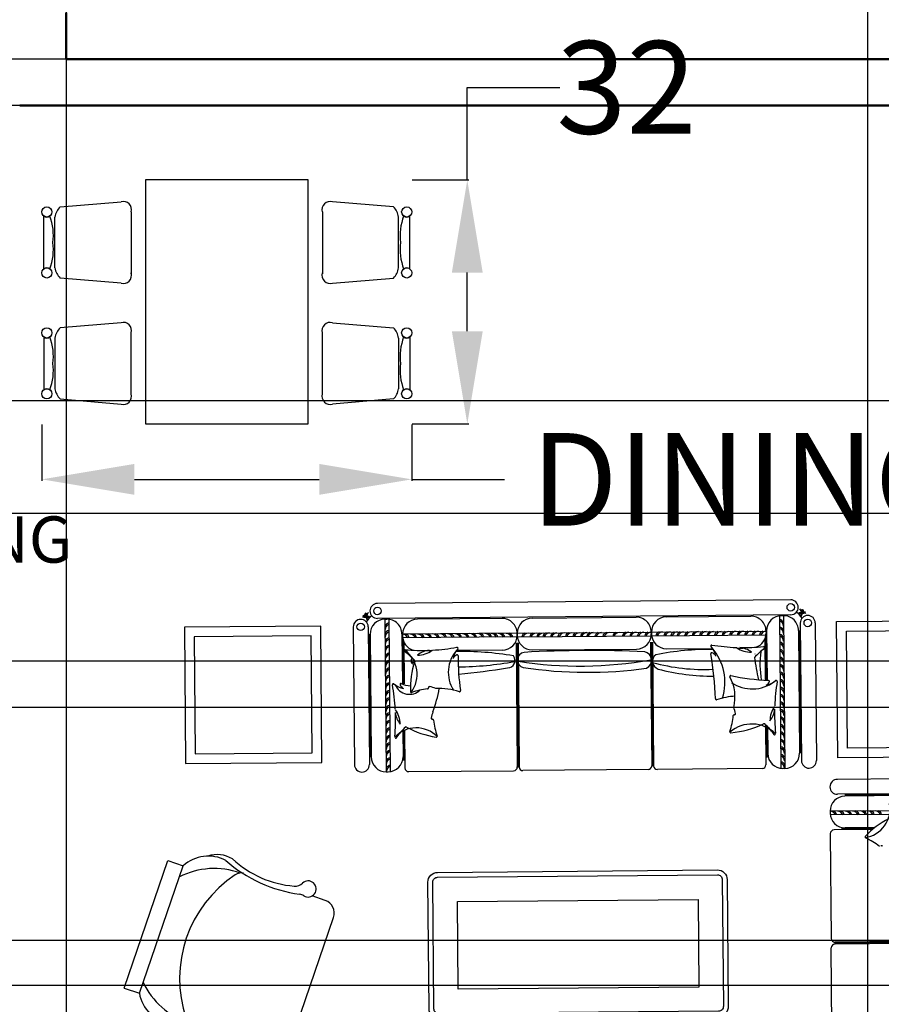
# Model space of a CAD drawing. Units: inches. Extents: x -77 to 516, y -119 to 536.
# Tile 8 of 11: x 224 to 335, y 159 to 287. Entities that reach past the tile are written whole.
import ezdxf

# ---------------------------------------------------------------- set-up
doc = ezdxf.new("R2010")
doc.units = ezdxf.units.IN
doc.header["$MEASUREMENT"] = 0
for name, color, linetype, lineweight in [('A-ANNO-DIMS', 2, 'Continuous', 18), ('A-AREA-IDEN', 170, 'Continuous', 25), ('furniture', 119, 'Continuous', 18), ('walls', 40, 'Continuous', 50)]:
    doc.layers.add(name, color=color, linetype=linetype, lineweight=lineweight)
doc.layers.add('FUR', color=42, linetype='Continuous')
doc.layers.add('ISLAK', color=6, linetype='Continuous')
doc.styles.get("Standard").update_dxf_attribs({"font": 'arial.ttf'})
doc.dimstyles.get("Standard").update_dxf_attribs({"dimtxt": 12, "dimasz": 12, "dimexe": 0.18, "dimexo": 0.0625, "dimgap": 0.09, "dimtad": 0, "dimtih": 1, "dimtoh": 1, "dimdec": 1, "dimzin": 0, "dimdsep": 46, "dimlunit": 4, "dimtxsty": 'Standard', "dimcen": 0.09, "dimadec": 0, "dimazin": 0, "dimtfac": 1, "dimtdec": 1, "dimtofl": 0, "dimtmove": 0, "dimatfit": 3, "dimfxl": 1, "dimtolj": 1, "dimtzin": 0, "dimarcsym": 0})

# ---------------------------------------------------------------- blocks, each defined once
blk = doc.blocks.new('A$C44A37715')
at = {"layer": 'FUR'}
for p, q in [((0.8644, 2.3252), (0.8644, 1.7873)), ((3.6462, 2.2614), (3.4159, 1.6094)), ((4.4156, 1.9896), (4.1853, 1.3376)), ((4.4938, 1.962), (4.4156, 1.9896)), ((4.4938, 1.962), (4.2635, 1.31)), ((0.2091, 1.7681), (0.8452, 1.7681)), ((0.2091, 1.7681), (0.8452, 1.7681)), ((0.2091, 1.7633), (0.8487, 1.7633)), ((0.2091, 1.7585), (0.8452, 1.7585)), ((0.2103, 1.7681), (0.8452, 1.7681)), ((0.8644, 1.2015), (0.8644, 1.7393)), ((3.4581, 1.5211), (3.5245, 1.4977)), ((4.2635, 1.31), (4.1853, 1.3376)), ((0.6364, 1.1727), (0.7875, 1.1727)), ((0.6445, 1.1775), (0.807, 1.1775)), ((0.6483, 1.1823), (0.8452, 1.1823)), ((0.5573, 1.0862), (0.8644, 1.0862)), ((0.56, 1.1054), (0.8638, 1.1054)), ((0.8644, 1.0862), (0.8644, 1.0958)), ((0.1193, 0.9998), (0.8259, 0.9998)), ((0.1577, 1.0094), (0.7875, 1.0094)), ((0.1577, 1.0046), (0.7875, 1.0046)), ((0.8644, 0.9614), (0.8644, 0.9614)), ((0.1193, 0.923), (0.8259, 0.923)), ((0.1193, 0.923), (0.8259, 0.923)), ((0.9706, 0.8644), (0.9706, 0.8644)), ((1.0954, 0.8644), (1.105, 0.8644)), ((1.0954, 0.0809), (1.0954, 0.8644)), ((1.1146, 0.0815), (1.1146, 0.8638)), ((1.2107, 0.8644), (1.7485, 0.8644)), ((1.7965, 0.8644), (2.438, 0.8644)), ((3.0239, 0.8644), (2.486, 0.8644)), ((3.1199, 0.0815), (3.1199, 0.8638)), ((3.1391, 0.8644), (3.1295, 0.8644)), ((3.1391, 0.0809), (3.1391, 0.8644)), ((3.264, 0.8644), (3.264, 0.8644)), ((0.9322, 0.1193), (0.9322, 0.8259)), ((1.009, 0.1193), (1.009, 0.8259)), ((1.1915, 0.6395), (1.1915, 0.8452)), ((1.7677, 0.2103), (1.7677, 0.8452)), ((1.7725, 0.2103), (1.7725, 0.8485)), ((1.7773, 0.2103), (1.7773, 0.8452)), ((2.4572, 0.2091), (2.4572, 0.8452)), ((2.4572, 0.2091), (2.4572, 0.8452)), ((2.462, 0.2091), (2.462, 0.8487)), ((2.4668, 0.2091), (2.4668, 0.8452)), ((3.0431, 0.652), (3.0431, 0.8452)), ((3.2255, 0.1193), (3.2255, 0.8259)), ((3.3024, 0.1193), (3.3024, 0.8259)), ((3.3024, 0.1193), (3.3024, 0.8259)), ((1.0138, 0.1577), (1.0138, 0.7875)), ((1.0186, 0.1577), (1.0186, 0.7875)), ((1.1819, 0.6496), (1.1819, 0.7875)), ((1.1867, 0.6445), (1.1867, 0.807)), ((3.0479, 0.6542), (3.0479, 0.807)), ((3.0527, 0.6565), (3.0527, 0.7875)), ((3.2159, 0.1577), (3.2159, 0.7875)), ((3.2207, 0.1577), (3.2207, 0.7875)), ((1.1819, 0.1577), (1.1819, 0.413)), ((1.1867, 0.1845), (1.1867, 0.4135)), ((1.1915, 0.1995), (1.1915, 0.4138)), ((3.0431, 0.1995), (3.0431, 0.4138)), ((3.0479, 0.1845), (3.0479, 0.4135)), ((3.0527, 0.1577), (3.0527, 0.413)), ((1.3318, 0.2455), (1.3038, 0.2455)), ((1.696, 0.2455), (1.4606, 0.2455)), ((2.3845, 0.2455), (1.8504, 0.2455)), ((2.5386, 0.2455), (2.774, 0.2455)), ((2.9027, 0.2455), (2.9308, 0.2455)), ((1.185, 0.1591), (1.185, 0.1687)), ((1.7728, 0.1591), (1.185, 0.1591)), ((1.7722, 0.1783), (1.1856, 0.1783)), ((1.7728, 0.1591), (1.7728, 0.1687)), ((1.7735, 0.1591), (1.7735, 0.1687)), ((2.4613, 0.1591), (1.7735, 0.1591)), ((2.4607, 0.1783), (1.7741, 0.1783)), ((2.4613, 0.1591), (2.4613, 0.1687)), ((2.4613, 0.1591), (2.4613, 0.1687)), ((2.4617, 0.1591), (2.4617, 0.1687)), ((2.4617, 0.1591), (2.4617, 0.1687)), ((2.4617, 0.1591), (3.0495, 0.1591)), ((2.4623, 0.1783), (3.0489, 0.1783)), ((2.4631, 0.1591), (2.4631, 0.1687)), ((3.0495, 0.1591), (3.0495, 0.1687)), ((0.9706, 0.0809), (0.9706, 0.0809)), ((1.0572, 0.0768), (3.1773, 0.0768)), ((1.0954, 0.0809), (1.105, 0.0809)), ((1.696, 0.0822), (1.2619, 0.0822)), ((2.3845, 0.0822), (1.8504, 0.0822)), ((2.5386, 0.0822), (2.9727, 0.0822)), ((3.1391, 0.0809), (3.1295, 0.0809)), ((3.264, 0.0809), (3.264, 0.0809)), ((1.0188, 0.0384), (1.0188, 0.0384)), ((1.0572, 0), (3.1773, 0)), ((3.2157, 0.0384), (3.2157, 0.0384))]:
    blk.add_line(p, q, dxfattribs=at)
for points in [[(2.8805, 2.1325, -0.414214), (2.9305, 2.0825), (2.9305, 1.4325, -0.414214), (2.8805, 1.3825), (1.4454, 1.3825, -0.414214), (1.3954, 1.4325), (1.3954, 2.0825, -0.414214), (1.4454, 2.1325)], [(2.8805, 2.1075, -0.414214), (2.9055, 2.0825), (2.9055, 1.4325, -0.414214), (2.8805, 1.4075), (1.4454, 1.4075, -0.414214), (1.4204, 1.4325), (1.4204, 2.0825, -0.414214), (1.4454, 2.1075)]]:
    blk.add_lwpolyline(points, format="xyb", close=True, dxfattribs=at)
for points in [[(2.7805, 1.9825), (2.7805, 1.5325), (1.5454, 1.5325), (1.5454, 1.9825)], [(0.1226, 0.1134), (0.1226, 0.8134), (0.8226, 0.8134), (0.8226, 0.1134)], [(4.1685, 0.1134), (4.1685, 0.8134), (3.4685, 0.8134), (3.4685, 0.1134)], [(0.1726, 0.1634), (0.1726, 0.7634), (0.7726, 0.7634), (0.7726, 0.1634)], [(4.1185, 0.1634), (4.1185, 0.7634), (3.5185, 0.7634), (3.5185, 0.1634)]]:
    blk.add_lwpolyline(points, close=True, dxfattribs=at)
for centre in [(0.9706, 0.1193), (3.264, 0.1193), (1.0572, 0.0384), (3.1773, 0.0384)]:
    blk.add_circle(centre, 0.0192, dxfattribs=at)
for centre, radius, start, end in [((4.0372, 1.7694), 0.3939, 24.5429, 71.319), ((4.2282, 1.96), 0.1897, 8.9926, 80.0637), ((3.5673, 1.9225), 0.6416, 303.2315, 17.8639), ((0.8452, 1.7873), 0.0192, 270, 0), ((0.8452, 1.7393), 0.0192, 0, 90), ((3.4811, 1.5863), 0.0691, 160.5477, 250.5477), ((3.5455, 1.4619), 0.0415, 57.5813, 313.2014), ((3.5974, 1.5436), 0.0553, 237.5813, 261.4346), ((3.4801, 0.7648), 0.7323, 48.4002, 81.4346), ((3.6117, 1.3913), 0.0553, 85.1896, 133.2014), ((3.5729, 0.9298), 0.5185, 46.2014, 85.1896), ((3.8886, 1.4321), 0.0553, 256.3156, 303.2315), ((4.0292, 1.7466), 0.3939, 249.7764, 296.5525), ((4.0581, 1.4783), 0.1897, 241.0317, 312.1028), ((0.6012, 1.2702), 0.0048, 215.4865, 326.8671), ((0.8574, 1.5872), 0.4019, 232.3976, 244.3894), ((4.0123, 1.437), 0.1555, 238.7962, 287.4358), ((0.7061, 1.0752), 0.1492, 97.8738, 190.1124), ((0.3864, 1.4953), 0.4082, 295.8111, 316.9977), ((0.6816, 1.2205), 0.0048, 313.302, 64.3894), ((0.7875, 1.0958), 0.0768, 0, 90), ((0.8452, 1.2015), 0.0192, 270, 0), ((0.6245, 1.1094), 0.0245, 189.3902, 251.5618), ((0.6348, 1.1155), 0.0293, 200.1355, 268.1936), ((0.6629, 1.1094), 0.0245, 189.3902, 251.5618), ((0.6732, 1.1155), 0.0293, 200.1355, 268.1936), ((0.7013, 1.1094), 0.0245, 189.3902, 251.5618), ((0.7116, 1.1155), 0.0293, 200.1355, 268.1936), ((0.7397, 1.1094), 0.0245, 189.3902, 251.5618), ((0.75, 1.1155), 0.0293, 200.1355, 268.1936), ((0.7781, 1.1094), 0.0245, 189.3902, 251.5618), ((0.7885, 1.1155), 0.0293, 200.1355, 268.1936), ((0.7875, 1.0862), 0.0768, 270, 0), ((0.8165, 1.1094), 0.0245, 189.3902, 251.5618), ((0.8269, 1.1155), 0.0293, 200.1355, 268.1936), ((0.8549, 1.1094), 0.0245, 189.3902, 251.5618), ((0.8653, 1.1155), 0.0293, 200.1355, 268.1936), ((0.8259, 0.9614), 0.0384, 360, 90), ((0.8259, 0.9614), 0.0384, 270, 360), ((0.9706, 0.8259), 0.0384, 90, 180), ((0.9706, 0.8259), 0.0384, 0, 90), ((1.0954, 0.7875), 0.0768, 90, 180), ((1.1247, 0.8653), 0.0293, 181.8064, 249.8645), ((1.105, 0.7875), 0.0768, 0, 90), ((1.2107, 0.8452), 0.0192, 90, 180), ((1.7485, 0.8452), 0.0192, 360, 90), ((1.7965, 0.8452), 0.0192, 90, 180), ((2.438, 0.8452), 0.0192, 0, 90), ((2.486, 0.8452), 0.0192, 90, 180), ((3.0239, 0.8452), 0.0192, 360, 90), ((3.1295, 0.7875), 0.0768, 90, 180), ((3.1098, 0.8653), 0.0293, 290.1355, 358.1936), ((3.1391, 0.7875), 0.0768, 360, 90), ((3.264, 0.8259), 0.0384, 90, 180), ((3.264, 0.8259), 0.0384, 360, 90), ((1.1186, 0.8549), 0.0245, 198.4382, 260.6098), ((1.1247, 0.8269), 0.0293, 181.8064, 249.8645), ((1.1186, 0.8165), 0.0245, 198.4382, 260.6098), ((3.1159, 0.8549), 0.0245, 279.3902, 341.5618), ((3.1098, 0.8269), 0.0293, 290.1355, 358.1936), ((3.1159, 0.8165), 0.0245, 279.3902, 341.5618), ((1.1247, 0.7885), 0.0293, 181.8064, 249.8645), ((1.1186, 0.7781), 0.0245, 198.4382, 260.6098), ((3.1098, 0.7885), 0.0293, 290.1355, 358.1936), ((3.1159, 0.7781), 0.0245, 279.3902, 341.5618), ((1.1247, 0.75), 0.0293, 181.8064, 249.8645), ((1.1186, 0.7397), 0.0245, 198.4382, 260.6098), ((1.1247, 0.7116), 0.0293, 181.8064, 249.8645), ((3.1098, 0.75), 0.0293, 290.1355, 358.1936), ((3.1159, 0.7397), 0.0245, 279.3902, 341.5618), ((3.1098, 0.7116), 0.0293, 290.1355, 358.1936), ((1.1186, 0.7013), 0.0245, 198.4382, 260.6098), ((1.1247, 0.6732), 0.0293, 181.8064, 249.8645), ((0.1462, 0.589), 0.9988, 358.3824, 5.4148), ((1.1462, 0.6869), 0.0048, 335.526, 185.4148), ((1.2637, 0.8067), 0.1714, 224.534, 310.2675), ((1.8739, 1.2944), 0.9459, 220.1216, 224.1481), ((1.4224, 0.1376), 0.5445, 95.5708, 113.9077), ((1.7562, 0.5476), 0.4019, 161.7886, 173.7804), ((1.3698, 0.6747), 0.0048, 341.7886, 92.876), ((2.8815, 0.6843), 0.0048, 87.124, 198.2114), ((2.9845, 0.7907), 0.1505, 224.349, 316.1606), ((2.4952, 0.5572), 0.4019, 6.2196, 18.2114), ((2.8036, 0.2306), 0.4652, 60.481, 80.3238), ((2.3606, 1.2944), 0.9459, 315.8519, 319.8784), ((3.0883, 0.6869), 0.0048, 354.5852, 204.474), ((4.0883, 0.589), 0.9988, 174.5852, 181.6176), ((3.1159, 0.7013), 0.0245, 279.3902, 341.5618), ((3.1098, 0.6732), 0.0293, 290.1355, 358.1936), ((1.1186, 0.6629), 0.0245, 198.4382, 260.6098), ((1.1247, 0.6348), 0.0293, 181.8064, 249.8645), ((1.1186, 0.6245), 0.0245, 198.4382, 260.6098), ((1.2514, 0.5519), 0.1071, 140.4453, 175.2684), ((1.0442, 0.6194), 0.1246, 323.9244, 0.3374), ((1.1986, 0.639), 0.0048, 224.1481, 310.8342), ((3.0359, 0.639), 0.0048, 229.1658, 315.8519), ((2.9831, 0.5519), 0.1071, 4.7316, 39.5547), ((3.1903, 0.6194), 0.1246, 179.6626, 216.0756), ((3.1159, 0.6629), 0.0245, 279.3902, 341.5618), ((3.1098, 0.6348), 0.0293, 290.1355, 358.1936), ((3.1159, 0.6245), 0.0245, 279.3902, 341.5618), ((1.1247, 0.5964), 0.0293, 181.8064, 249.8645), ((1.1186, 0.586), 0.0245, 198.4382, 260.6098), ((1.1247, 0.558), 0.0293, 181.8064, 249.8645), ((1.3501, 0.5822), 0.0048, 79.311, 190.6915), ((1.5338, 0.6169), 0.1918, 190.6915, 200.5832), ((1.3518, 0.5916), 0.0048, 259.311, 353.7804), ((3.5654, 0.3102), 0.7132, 159.5737, 169.6301), ((2.8995, 0.6013), 0.0048, 186.2196, 280.689), ((2.7176, 0.6265), 0.1918, 339.4168, 349.3085), ((2.9013, 0.5918), 0.0048, 349.3085, 100.689), ((3.1098, 0.5964), 0.0293, 290.1355, 358.1936), ((3.1159, 0.586), 0.0245, 279.3902, 341.5618), ((3.1098, 0.558), 0.0293, 290.1355, 358.1936), ((1.1186, 0.5476), 0.0245, 198.4382, 260.6098), ((1.1247, 0.5195), 0.0293, 181.8064, 249.8645), ((0.1462, 0.589), 0.9988, 350.147, 357.3879), ((1.5642, 0.4939), 0.2171, 165.1637, 207.9713), ((1.3224, 0.8929), 0.4019, 273.5087, 287.2752), ((1.4432, 0.5045), 0.0048, 349.041, 107.2752), ((4.0883, 0.589), 0.9988, 182.6121, 189.853), ((3.1159, 0.5476), 0.0245, 279.3902, 341.5618), ((3.1098, 0.5195), 0.0293, 290.1355, 358.1936), ((1.1186, 0.5092), 0.0245, 198.4382, 260.6098), ((1.1247, 0.4811), 0.0293, 181.8064, 249.8645), ((1.1186, 0.4708), 0.0245, 198.4382, 260.6098), ((1.257, 0.2644), 0.191, 55.8675, 126.0186), ((1.6647, 0.4171), 0.2669, 161.6936, 220.7721), ((3.108, 0.5412), 1.6605, 181.2996, 189.2908), ((2.759, 0.4518), 0.0048, 72.7248, 190.959), ((2.8798, 0.8402), 0.4019, 252.7248, 270.2702), ((2.8798, 0.8402), 0.4019, 276.2196, 288.2114), ((3.0162, 0.388), 0.0798, 22.7628, 133.8922), ((3.1333, 0.3647), 0.1565, 143.1921, 233.1518), ((3.0069, 0.4538), 0.0048, 357.124, 108.2114), ((3.1159, 0.5092), 0.0245, 279.3902, 341.5618), ((3.1098, 0.4811), 0.0293, 290.1355, 358.1936), ((3.1159, 0.4708), 0.0245, 279.3902, 341.5618), ((1.1247, 0.4427), 0.0293, 181.8064, 249.8645), ((1.1186, 0.4324), 0.0245, 198.4382, 260.6098), ((1.1351, 0.4172), 0.0048, 170.147, 311.7497), ((1.2047, 0.3392), 0.0998, 100.2155, 131.7497), ((1.1745, 0.417), 0.0048, 161.7015, 277.2637), ((1.2, 0.4085), 0.0317, 114.2109, 161.7015), ((1.1136, -0.7491), 1.1629, 77.4179, 86.9678), ((0.7221, 0.3308), 0.4956, 352.2178, 9.1534), ((0.0106, 0.1327), 1.2458, 7.4166, 12.7868), ((1.7817, 0.3017), 0.984, 358.3396, 8.7219), ((2.646, 0.358), 0.1707, 317.5546, 31.9076), ((2.9491, 0.6178), 0.1918, 249.4168, 259.3085), ((2.9144, 0.4341), 0.0048, 259.3085, 10.689), ((2.9238, 0.4358), 0.0048, 96.2196, 190.689), ((2.574, 0.4412), 0.4378, 341.1597, 1.6138), ((2.9856, 0.2241), 0.2021, 68.5609, 82.62), ((3.0298, 0.3392), 0.0998, 48.2503, 79.7845), ((3.0345, 0.4085), 0.0317, 18.2985, 65.7891), ((3.0601, 0.417), 0.0048, 262.7363, 18.2985), ((3.0995, 0.4172), 0.0048, 228.2503, 9.853), ((3.1098, 0.4427), 0.0293, 290.1355, 358.1936), ((3.1159, 0.4324), 0.0245, 279.3902, 341.5618), ((1.1247, 0.4043), 0.0293, 181.8064, 249.8645), ((1.1186, 0.394), 0.0245, 198.4382, 260.6098), ((1.1247, 0.3659), 0.0293, 181.8064, 249.8645), ((1.3678, 0.3906), 0.0048, 259.041, 17.2752), ((1.452, -0.6985), 1.0865, 74.5837, 89.8632), ((2.0845, -1.8144), 2.1772, 80.8163, 97.5183), ((3.1491, -3.8439), 4.2285, 95.2294, 98.6658), ((3.1098, 0.4043), 0.0293, 290.1355, 358.1936), ((3.1159, 0.394), 0.0245, 279.3902, 341.5618), ((3.1098, 0.3659), 0.0293, 290.1355, 358.1936), ((1.1186, 0.3555), 0.0245, 198.4382, 260.6098), ((1.1247, 0.3275), 0.0293, 181.8064, 249.8645), ((1.1186, 0.3171), 0.0245, 198.4382, 260.6098), ((1.4976, -0.6222), 0.9756, 73.912, 92.3145), ((1.7263, 0.3094), 0.0421, 306.2374, 69.8277), ((1.8184, 0.3033), 0.045, 114.6729, 256.8791), ((2.1234, -1.693), 2.0235, 80.5045, 99.8273), ((2.4224, 0.2967), 0.0394, 276.868, 75.9734), ((2.512, 0.2984), 0.0379, 90.0798, 217.436), ((2.7657, -1.375), 1.7039, 90.0689, 99.7358), ((2.7556, -0.7438), 1.0743, 76.4982, 77.2888), ((2.988, 0.2957), 0.0192, 312.662, 59.1573), ((3.1159, 0.3555), 0.0245, 279.3902, 341.5618), ((3.1098, 0.3275), 0.0293, 290.1355, 358.1936), ((3.1159, 0.3171), 0.0245, 279.3902, 341.5618), ((1.1247, 0.289), 0.0293, 181.8064, 249.8645), ((1.1186, 0.2787), 0.0245, 198.4382, 260.6098), ((0.587, 0.972), 0.9459, 309.9755, 314.1671), ((1.4789, 1.3249), 1.0743, 257.2794, 257.2982), ((1.2621, 0.1423), 0.1246, 53.9244, 90.3374), ((1.3295, 0.3495), 0.1071, 230.4453, 265.2684), ((1.5423, 0.3028), 0.0998, 190.2155, 221.7497), ((1.473, 0.2981), 0.0317, 204.2109, 251.7015), ((1.4827, 1.717), 1.4665, 269.0007, 280.5511), ((1.4645, 0.2725), 0.0048, 251.7015, 7.2637), ((2.1367, 6.3553), 6.1046, 266.91491, 272.72666), ((2.7517, 1.731), 1.4804, 259.4989, 270.9947), ((2.77, 0.2725), 0.0048, 172.7363, 288.2985), ((2.6923, 0.3028), 0.0998, 318.2503, 349.7845), ((2.7616, 0.2981), 0.0317, 288.2985, 335.7891), ((2.9725, 0.1423), 0.1246, 89.6626, 126.0756), ((2.905, 0.3495), 0.1071, 274.7316, 309.5547), ((2.992, 0.2967), 0.0048, 139.1658, 225.8519), ((3.6475, 0.972), 0.9459, 225.8519, 230.0245), ((3.1098, 0.289), 0.0293, 290.1355, 358.1936), ((3.1159, 0.2787), 0.0245, 279.3902, 341.5618), ((1.1247, 0.2506), 0.0293, 181.8064, 249.8645), ((1.1186, 0.2403), 0.0245, 198.4382, 260.6098), ((1.1247, 0.2122), 0.0293, 181.8064, 249.8645), ((1.2619, 0.1687), 0.0768, 108.3026, 180), ((1.1978, 0.2435), 0.0048, 129.9755, 275.4148), ((1.2925, -0.7557), 0.9988, 88.3824, 95.4148), ((1.3382, 0.2469), 0.0048, 233.9244, 267.3879), ((1.2925, -0.7557), 0.9988, 80.147, 87.3879), ((1.4642, 0.2331), 0.0048, 260.147, 41.7497), ((1.696, 0.1687), 0.0768, 0, 90), ((1.8504, 0.1687), 0.0768, 90, 180), ((2.3845, 0.1687), 0.0768, 0, 90), ((2.5386, 0.1687), 0.0768, 90, 180), ((2.7703, 0.2331), 0.0048, 138.2503, 279.853), ((2.942, -0.7557), 0.9988, 92.6121, 99.853), ((2.942, -0.7557), 0.9988, 84.5852, 91.6176), ((2.9727, 0.1687), 0.0768, 360, 71.6974), ((3.0367, 0.2435), 0.0048, 264.5852, 50.0245), ((3.1098, 0.2506), 0.0293, 290.1355, 358.1936), ((3.1159, 0.2403), 0.0245, 279.3902, 341.5618), ((3.1098, 0.2122), 0.0293, 290.1355, 358.1936), ((1.0954, 0.1577), 0.0768, 180, 270), ((1.1186, 0.2019), 0.0245, 198.4382, 260.6098), ((1.1247, 0.1738), 0.0293, 181.8064, 249.8645), ((1.1186, 0.1635), 0.0245, 198.4382, 260.6098), ((1.105, 0.1577), 0.0768, 270, 0), ((1.1841, 0.1884), 0.0293, 271.8064, 339.8645), ((1.2619, 0.1591), 0.0768, 180, 270), ((1.1944, 0.1823), 0.0245, 288.4382, 350.6098), ((1.2225, 0.1884), 0.0293, 271.8064, 339.8645), ((1.2329, 0.1823), 0.0245, 288.4382, 350.6098), ((1.2609, 0.1884), 0.0293, 271.8064, 339.8645), ((1.2713, 0.1823), 0.0245, 288.4382, 350.6098), ((1.2994, 0.1884), 0.0293, 271.8064, 339.8645), ((1.3097, 0.1823), 0.0245, 288.4382, 350.6098), ((1.3378, 0.1884), 0.0293, 271.8064, 339.8645), ((1.3481, 0.1823), 0.0245, 288.4382, 350.6098), ((1.3762, 0.1884), 0.0293, 271.8064, 339.8645), ((1.3865, 0.1823), 0.0245, 288.4382, 350.6098), ((1.4146, 0.1884), 0.0293, 271.8064, 339.8645), ((1.4249, 0.1823), 0.0245, 288.4382, 350.6098), ((1.453, 0.1884), 0.0293, 271.8064, 339.8645), ((1.4633, 0.1823), 0.0245, 288.4382, 350.6098), ((1.4914, 0.1884), 0.0293, 271.8064, 339.8645), ((1.5018, 0.1823), 0.0245, 288.4382, 350.6098), ((1.5298, 0.1884), 0.0293, 271.8064, 339.8645), ((1.5402, 0.1823), 0.0245, 288.4382, 350.6098), ((1.5683, 0.1884), 0.0293, 271.8064, 339.8645), ((1.5786, 0.1823), 0.0245, 288.4382, 350.6098), ((1.6067, 0.1884), 0.0293, 271.8064, 339.8645), ((1.617, 0.1823), 0.0245, 288.4382, 350.6098), ((1.6386, 0.1884), 0.0293, 271.8064, 339.8645), ((1.649, 0.1823), 0.0245, 288.4382, 350.6098), ((1.6745, 0.1884), 0.0293, 271.8064, 339.8645), ((1.6848, 0.1823), 0.0245, 288.4382, 350.6098), ((1.696, 0.1591), 0.0768, 270, 0), ((1.7155, 0.1884), 0.0293, 271.8064, 339.8645), ((1.7258, 0.1823), 0.0245, 288.4382, 350.6098), ((1.7726, 0.1884), 0.0293, 271.8064, 339.8645), ((1.8504, 0.1591), 0.0768, 180, 270), ((1.783, 0.1823), 0.0245, 288.4382, 350.6098), ((1.811, 0.1884), 0.0293, 271.8064, 339.8645), ((1.8214, 0.1823), 0.0245, 288.4382, 350.6098), ((1.8495, 0.1884), 0.0293, 271.8064, 339.8645), ((1.8598, 0.1823), 0.0245, 288.4382, 350.6098), ((1.8879, 0.1884), 0.0293, 271.8064, 339.8645), ((1.8982, 0.1823), 0.0245, 288.4382, 350.6098), ((1.9369, 0.1884), 0.0293, 271.8064, 339.8645), ((1.9472, 0.1823), 0.0245, 288.4382, 350.6098), ((1.9873, 0.1884), 0.0293, 271.8064, 339.8645), ((1.9976, 0.1823), 0.0245, 288.4382, 350.6098), ((2.028, 0.1884), 0.0293, 271.8064, 339.8645), ((2.0384, 0.1823), 0.0245, 288.4382, 350.6098), ((2.0708, 0.1884), 0.0293, 271.8064, 339.8645), ((2.0812, 0.1823), 0.0245, 288.4382, 350.6098), ((2.1031, 0.1884), 0.0293, 271.8064, 339.8645), ((2.1135, 0.1823), 0.0245, 288.4382, 350.6098), ((2.1415, 0.1884), 0.0293, 271.8064, 339.8645), ((2.1519, 0.1823), 0.0245, 288.4382, 350.6098), ((2.18, 0.1884), 0.0293, 271.8064, 339.8645), ((2.1903, 0.1823), 0.0245, 288.4382, 350.6098), ((2.2184, 0.1884), 0.0293, 271.8064, 339.8645), ((2.2287, 0.1823), 0.0245, 288.4382, 350.6098), ((2.2568, 0.1884), 0.0293, 271.8064, 339.8645), ((2.2671, 0.1823), 0.0245, 288.4382, 350.6098), ((2.2952, 0.1884), 0.0293, 271.8064, 339.8645), ((2.3055, 0.1823), 0.0245, 288.4382, 350.6098), ((2.3272, 0.1884), 0.0293, 271.8064, 339.8645), ((2.3375, 0.1823), 0.0245, 288.4382, 350.6098), ((2.363, 0.1884), 0.0293, 271.8064, 339.8645), ((2.3733, 0.1823), 0.0245, 288.4382, 350.6098), ((2.3845, 0.1591), 0.0768, 270, 0), ((2.404, 0.1884), 0.0293, 271.8064, 339.8645), ((2.4143, 0.1823), 0.0245, 288.4382, 350.6098), ((2.5386, 0.1591), 0.0768, 180, 270), ((2.5087, 0.1823), 0.0245, 189.3902, 251.5618), ((2.5191, 0.1884), 0.0293, 200.1355, 268.1936), ((2.5497, 0.1823), 0.0245, 189.3902, 251.5618), ((2.5601, 0.1884), 0.0293, 200.1355, 268.1936), ((2.5856, 0.1823), 0.0245, 189.3902, 251.5618), ((2.5959, 0.1884), 0.0293, 200.1355, 268.1936), ((2.6175, 0.1823), 0.0245, 189.3902, 251.5618), ((2.6278, 0.1884), 0.0293, 200.1355, 268.1936), ((2.6559, 0.1823), 0.0245, 189.3902, 251.5618), ((2.6663, 0.1884), 0.0293, 200.1355, 268.1936), ((2.6943, 0.1823), 0.0245, 189.3902, 251.5618), ((2.7047, 0.1884), 0.0293, 200.1355, 268.1936), ((2.7328, 0.1823), 0.0245, 189.3902, 251.5618), ((2.7431, 0.1884), 0.0293, 200.1355, 268.1936), ((2.7712, 0.1823), 0.0245, 189.3902, 251.5618), ((2.7815, 0.1884), 0.0293, 200.1355, 268.1936), ((2.8096, 0.1823), 0.0245, 189.3902, 251.5618), ((2.8199, 0.1884), 0.0293, 200.1355, 268.1936), ((2.848, 0.1823), 0.0245, 189.3902, 251.5618), ((2.8583, 0.1884), 0.0293, 200.1355, 268.1936), ((2.8864, 0.1823), 0.0245, 189.3902, 251.5618), ((2.8968, 0.1884), 0.0293, 200.1355, 268.1936), ((2.9248, 0.1823), 0.0245, 189.3902, 251.5618), ((2.9352, 0.1884), 0.0293, 200.1355, 268.1936), ((2.9633, 0.1823), 0.0245, 189.3902, 251.5618), ((2.9736, 0.1884), 0.0293, 200.1355, 268.1936), ((2.9727, 0.1591), 0.0768, 270, 360), ((3.0017, 0.1823), 0.0245, 189.3902, 251.5618), ((3.012, 0.1884), 0.0293, 200.1355, 268.1936), ((3.0401, 0.1823), 0.0245, 189.3902, 251.5618), ((3.0504, 0.1884), 0.0293, 200.1355, 268.1936), ((3.1295, 0.1577), 0.0768, 180, 270), ((3.1159, 0.2019), 0.0245, 279.3902, 341.5618), ((3.1098, 0.1738), 0.0293, 290.1355, 358.1936), ((3.1159, 0.1635), 0.0245, 279.3902, 341.5618), ((3.1391, 0.1577), 0.0768, 270, 360), ((0.9706, 0.1193), 0.0384, 180, 270), ((0.9706, 0.1193), 0.0384, 270, 360), ((1.1247, 0.1354), 0.0293, 181.8064, 249.8645), ((1.1186, 0.125), 0.0245, 198.4382, 260.6098), ((3.1098, 0.1354), 0.0293, 290.1355, 358.1936), ((3.1159, 0.125), 0.0245, 279.3902, 341.5618), ((3.264, 0.1193), 0.0384, 180, 270), ((3.264, 0.1193), 0.0384, 270, 360), ((0.9923, 0.0778), 0.0137, 207.9368, 312.4811), ((0.9943, 0.0576), 0.0124, 54.0121, 169.8317), ((1.0004, 0.0585), 0.00925, 82.5827, 252.2087), ((1.0033, 0.0606), 0.00723, 104.0764, 299.9545), ((1.0016, 0.0466), 0.00508, 39.2756, 143.3144), ((1.0085, 0.0743), 0.0096, 99.0044, 348.6149), ((1.0954, 0.1577), 0.1152, 213.5982, 234.4891), ((1.0304, 0.0673), 0.0288, 179.3374, 226.5372), ((1.009, 0.075), 0.0048, 69.1702, 18.3087), ((1.0572, 0.0384), 0.0384, 90, 180), ((3.1773, 0.0384), 0.0384, 0, 90), ((3.1391, 0.1577), 0.1152, 305.5109, 326.4018), ((3.226, 0.0743), 0.0096, 191.3851, 80.9956), ((3.2255, 0.075), 0.0048, 161.6913, 110.8298), ((3.2042, 0.0673), 0.0288, 313.4628, 0.6626), ((3.2312, 0.0606), 0.00723, 240.0455, 75.9236), ((3.2329, 0.0466), 0.00508, 36.6856, 140.7244), ((3.2422, 0.0778), 0.0137, 227.5189, 332.0632), ((3.2403, 0.0576), 0.0124, 10.1683, 125.9879), ((3.2342, 0.0585), 0.00925, 287.7913, 97.4173), ((1.0572, 0.0384), 0.0384, 180, 270), ((3.1773, 0.0384), 0.0384, 270, 0)]:
    blk.add_arc(centre, radius, start, end, dxfattribs=at)
blk = doc.blocks.new('A$C34D4650F')
at = {"layer": 'ISLAK'}
for p, q in [((0.4, 0), (-0.4, 0)), ((-0.4, 0), (-0.4, -1.2)), ((0.4, -1.2), (0.4, 0)), ((-0.82, -0.1325), (-0.52, -0.1075)), ((0.82, -0.1325), (0.52, -0.1075)), ((-0.9, -0.3075), (-0.9, -0.1775)), ((-0.845, -0.3075), (-0.845, -0.1825)), ((-0.47, -0.1575), (-0.47, -0.4625)), ((0.47, -0.1575), (0.47, -0.4625)), ((0.845, -0.3075), (0.845, -0.1825)), ((0.9, -0.3075), (0.9, -0.1775)), ((-0.9, -0.4375), (-0.9, -0.3075)), ((-0.845, -0.4325), (-0.845, -0.3075)), ((0.845, -0.4325), (0.845, -0.3075)), ((0.9, -0.4375), (0.9, -0.3075)), ((-0.52, -0.5075), (-0.82, -0.4825)), ((0.52, -0.5075), (0.82, -0.4825)), ((-0.52, -0.7025), (-0.82, -0.7275)), ((0.52, -0.7025), (0.82, -0.7275)), ((-0.9, -0.7725), (-0.9, -0.9025)), ((-0.47, -1.0525), (-0.47, -0.7475)), ((0.47, -1.0525), (0.47, -0.7475)), ((0.9, -0.7725), (0.9, -0.9025)), ((-0.845, -0.7775), (-0.845, -0.9025)), ((0.845, -0.7775), (0.845, -0.9025)), ((-0.9, -0.9025), (-0.9, -1.0325)), ((-0.845, -0.9025), (-0.845, -1.0275)), ((0.845, -0.9025), (0.845, -1.0275)), ((0.9, -0.9025), (0.9, -1.0325)), ((-0.82, -1.0775), (-0.52, -1.1025)), ((0.82, -1.0775), (0.52, -1.1025)), ((-0.4, -1.2), (0.4, -1.2))]:
    blk.add_line(p, q, dxfattribs=at)
for centre in [(-0.885, -0.1575), (0.885, -0.1575), (-0.885, -0.4575), (0.885, -0.4575), (-0.885, -0.7525), (0.885, -0.7525), (-0.885, -1.0525), (0.885, -1.0525)]:
    blk.add_circle(centre, 0.025, dxfattribs=at)
for centre, radius, start, end in [((-0.7575, -0.195), 0.0884, 135, 171.8699), ((-0.5083, -0.1458), 0.0401, 343.0725, 106.9275), ((0.5083, -0.1458), 0.0401, 73.0725, 196.9275), ((0.7575, -0.195), 0.0884, 8.1301, 45), ((-0.885, -0.1575), 0.025, 233.1301, 306.8699), ((-1.1225, -0.2725), 0.2698, 352.5457, 20.6182), ((1.1225, -0.2725), 0.2698, 159.3818, 187.4543), ((0.885, -0.1575), 0.025, 233.1301, 306.8699), ((-1.1225, -0.3425), 0.2698, 339.3818, 7.4543), ((1.1225, -0.3425), 0.2698, 172.5457, 200.6182), ((-0.885, -0.4575), 0.025, 53.1301, 126.8699), ((-0.7575, -0.42), 0.0884, 188.1301, 225), ((0.7575, -0.42), 0.0884, 315, 351.8699), ((0.885, -0.4575), 0.025, 53.1301, 126.8699), ((-0.5083, -0.4692), 0.0401, 253.0725, 16.9275), ((0.5083, -0.4692), 0.0401, 163.0725, 286.9275), ((-0.5083, -0.7408), 0.0401, 343.0725, 106.9275), ((0.5083, -0.7408), 0.0401, 73.0725, 196.9275), ((-0.885, -0.7525), 0.025, 233.1301, 306.8699), ((-1.1225, -0.8675), 0.2698, 352.5457, 20.6182), ((-0.7575, -0.79), 0.0884, 135, 171.8699), ((0.7575, -0.79), 0.0884, 8.1301, 45), ((1.1225, -0.8675), 0.2698, 159.3818, 187.4543), ((0.885, -0.7525), 0.025, 233.1301, 306.8699), ((-1.1225, -0.9375), 0.2698, 339.3818, 7.4543), ((1.1225, -0.9375), 0.2698, 172.5457, 200.6182), ((-0.885, -1.0525), 0.025, 53.1301, 126.8699), ((-0.7575, -1.015), 0.0884, 188.1301, 225), ((-0.5083, -1.0642), 0.0401, 253.0725, 16.9275), ((0.5083, -1.0642), 0.0401, 163.0725, 286.9275), ((0.7575, -1.015), 0.0884, 315, 351.8699), ((0.885, -1.0525), 0.025, 53.1301, 126.8699)]:
    blk.add_arc(centre, radius, start, end, dxfattribs=at)
blk = doc.blocks.new('*D32')
at = {"layer": 'A-ANNO-DIMS', "color": 0, "lineweight": -2, "transparency": 16777216}
for p, q in [((226.61, 234.25), (226.61, 226.94)), ((274.55, 234.25), (274.55, 226.94)), ((238.61, 227.12), (262.55, 227.12)), ((274.55, 227.12), (286.55, 227.12))]:
    blk.add_line(p, q, dxfattribs=at)
at = {"layer": 'A-ANNO-DIMS', "color": 0, "transparency": 16777216}
for points in [[(238.61, 229.12), (238.61, 225.12), (226.61, 227.12)], [(262.55, 229.12), (262.55, 225.12), (274.55, 227.12)]]:
    blk.add_solid(points, dxfattribs=at)
at = {"layer": 'Defpoints', "color": 0, "transparency": 16777216}
for p in [(226.61, 234.31), (274.55, 234.31), (274.55, 227.12)]:
    blk.add_point(p, dxfattribs=at)
at = {"layer": 'A-ANNO-DIMS', "color": 0, "transparency": 16777216, "insert": (345.24, 227.12), "char_height": 12, "attachment_point": 5}
blk.add_mtext('\\A1;DINING SET 48', dxfattribs=at)
blk = doc.blocks.new('*D33')
at = {"layer": 'A-ANNO-DIMS', "color": 0, "lineweight": -2, "transparency": 16777216}
for p, q in [((281.74, 265.92), (281.74, 277.92)), ((281.74, 277.92), (293.74, 277.92)), ((274.61, 265.92), (281.92, 265.92)), ((281.74, 246.31), (281.74, 253.92)), ((274.61, 234.31), (281.92, 234.31))]:
    blk.add_line(p, q, dxfattribs=at)
at = {"layer": 'A-ANNO-DIMS', "color": 0, "transparency": 16777216}
for points in [[(279.74, 253.92), (283.74, 253.92), (281.74, 265.92)], [(279.74, 246.31), (283.74, 246.31), (281.74, 234.31)]]:
    blk.add_solid(points, dxfattribs=at)
at = {"layer": 'Defpoints', "color": 0, "transparency": 16777216}
for p in [(274.55, 265.92), (281.74, 265.92), (274.55, 234.31)]:
    blk.add_point(p, dxfattribs=at)
at = {"layer": 'A-ANNO-DIMS', "color": 0, "transparency": 16777216, "insert": (302.36, 277.92), "char_height": 12, "attachment_point": 5}
blk.add_mtext('\\A1;32', dxfattribs=at)
blk = doc.blocks.new('*D37')
at = {"layer": 'A-ANNO-DIMS', "color": 0, "lineweight": -2, "transparency": 16777216}
for p, q in [((373.81, 494.59), (454.58, 494.59)), ((454.4, 482.59), (454.4, 212.81)), ((454.4, -69.41), (454.4, 200.37)), ((309, -81.41), (454.58, -81.41))]:
    blk.add_line(p, q, dxfattribs=at)
at = {"layer": 'A-ANNO-DIMS', "color": 0, "transparency": 16777216}
for points in [[(452.4, 482.59), (456.4, 482.59), (454.4, 494.59)], [(452.4, -69.41), (456.4, -69.41), (454.4, -81.41)]]:
    blk.add_solid(points, dxfattribs=at)
at = {"layer": 'Defpoints', "color": 0, "transparency": 16777216}
for p in [(373.75, 494.59), (454.4, 494.59), (308.93, -81.41)]:
    blk.add_point(p, dxfattribs=at)
at = {"layer": 'A-ANNO-DIMS', "color": 0, "transparency": 16777216, "insert": (454.4, 206.59), "char_height": 12, "attachment_point": 5}
blk.add_mtext('\\A1;576', dxfattribs=at)
blk = doc.blocks.new('*D41')
at = {"layer": 'A-ANNO-DIMS', "color": 0, "lineweight": -2, "transparency": 16777216}
for p, q in [((229.75, 485.53), (229.75, -111.24)), ((333.59, 485.53), (333.59, -111.24)), ((241.75, -111.06), (257.26, -111.06)), ((321.59, -111.06), (306.08, -111.06))]:
    blk.add_line(p, q, dxfattribs=at)
at = {"layer": 'A-ANNO-DIMS', "color": 0, "transparency": 16777216}
for points in [[(241.75, -109.06), (241.75, -113.06), (229.75, -111.06)], [(321.59, -109.06), (321.59, -113.06), (333.59, -111.06)]]:
    blk.add_solid(points, dxfattribs=at)
at = {"layer": 'Defpoints', "color": 0, "transparency": 16777216}
for p in [(229.75, 485.59), (333.59, 485.59), (333.59, -111.06)]:
    blk.add_point(p, dxfattribs=at)
at = {"layer": 'A-ANNO-DIMS', "color": 0, "transparency": 16777216, "insert": (281.67, -111.06), "char_height": 12, "attachment_point": 5}
blk.add_mtext('\\A1;103.84', dxfattribs=at)
blk = doc.blocks.new('*D42')
at = {"layer": 'A-ANNO-DIMS', "color": 0, "lineweight": -2, "transparency": 16777216}
for p, q in [((454.4, 197.59), (454.4, 209.59)), ((454.4, 209.59), (466.4, 209.59)), ((22.81, 197.59), (454.58, 197.59)), ((454.4, 179.41), (454.4, 185.59)), ((22.81, 167.41), (454.58, 167.41))]:
    blk.add_line(p, q, dxfattribs=at)
at = {"layer": 'A-ANNO-DIMS', "color": 0, "transparency": 16777216}
for points in [[(452.4, 185.59), (456.4, 185.59), (454.4, 197.59)], [(452.4, 179.41), (456.4, 179.41), (454.4, 167.41)]]:
    blk.add_solid(points, dxfattribs=at)
at = {"layer": 'Defpoints', "color": 0, "transparency": 16777216}
for p in [(22.75, 197.59), (454.4, 197.59), (22.75, 167.41)]:
    blk.add_point(p, dxfattribs=at)
at = {"layer": 'A-ANNO-DIMS', "color": 0, "transparency": 16777216, "insert": (486.75, 209.59), "char_height": 12, "attachment_point": 5}
blk.add_mtext('\\A1;30.18', dxfattribs=at)
blk = doc.blocks.new('*D43')
at = {"layer": 'A-ANNO-DIMS', "color": 0, "lineweight": -2, "transparency": 16777216}
for p, q in [((454.4, 237.36), (454.4, 249.36)), ((454.4, 249.36), (466.4, 249.36)), ((22.81, 237.36), (454.58, 237.36)), ((454.4, 215.59), (454.4, 225.36)), ((22.81, 203.59), (454.58, 203.59))]:
    blk.add_line(p, q, dxfattribs=at)
at = {"layer": 'A-ANNO-DIMS', "color": 0, "transparency": 16777216}
for points in [[(452.4, 225.36), (456.4, 225.36), (454.4, 237.36)], [(452.4, 215.59), (456.4, 215.59), (454.4, 203.59)]]:
    blk.add_solid(points, dxfattribs=at)
at = {"layer": 'Defpoints', "color": 0, "transparency": 16777216}
for p in [(22.75, 237.36), (454.4, 237.36), (22.75, 203.59)]:
    blk.add_point(p, dxfattribs=at)
at = {"layer": 'A-ANNO-DIMS', "color": 0, "transparency": 16777216, "insert": (491.44, 249.36), "char_height": 12, "attachment_point": 5}
blk.add_mtext('\\A1;33.775', dxfattribs=at)
blk = doc.blocks.new('*D47')
at = {"layer": 'A-ANNO-DIMS', "color": 0, "lineweight": -2, "transparency": 16777216}
for p, q in [((364.69, 275.59), (-16.08, 275.59)), ((-15.9, 263.59), (-15.9, 255.37)), ((-15.9, 234.71), (-15.9, 242.93)), ((364.69, 222.71), (-16.08, 222.71))]:
    blk.add_line(p, q, dxfattribs=at)
at = {"layer": 'A-ANNO-DIMS', "color": 0, "transparency": 16777216}
for points in [[(-17.9, 263.59), (-13.9, 263.59), (-15.9, 275.59)], [(-17.9, 234.71), (-13.9, 234.71), (-15.9, 222.71)]]:
    blk.add_solid(points, dxfattribs=at)
at = {"layer": 'Defpoints', "color": 0, "transparency": 16777216}
for p in [(-15.9, 275.59), (364.75, 275.59), (364.75, 222.71)]:
    blk.add_point(p, dxfattribs=at)
at = {"layer": 'A-ANNO-DIMS', "color": 0, "transparency": 16777216, "insert": (-15.9, 249.15), "char_height": 12, "attachment_point": 5}
blk.add_mtext('\\A1;52.87', dxfattribs=at)
blk = doc.blocks.new('*D48')
at = {"layer": 'A-ANNO-DIMS', "color": 0, "lineweight": -2, "transparency": 16777216}
for p, q in [((364.69, 323.24), (-16.08, 323.24)), ((-15.9, 311.24), (-15.9, 308.63)), ((-15.9, 293.59), (-15.9, 296.2)), ((364.69, 281.59), (-16.08, 281.59))]:
    blk.add_line(p, q, dxfattribs=at)
at = {"layer": 'A-ANNO-DIMS', "color": 0, "transparency": 16777216}
for points in [[(-17.9, 311.24), (-13.9, 311.24), (-15.9, 323.24)], [(-17.9, 293.59), (-13.9, 293.59), (-15.9, 281.59)]]:
    blk.add_solid(points, dxfattribs=at)
at = {"layer": 'Defpoints', "color": 0, "transparency": 16777216}
for p in [(-15.9, 323.24), (364.75, 323.24), (364.75, 281.59)]:
    blk.add_point(p, dxfattribs=at)
at = {"layer": 'A-ANNO-DIMS', "color": 0, "transparency": 16777216, "insert": (-15.9, 302.42), "char_height": 12, "attachment_point": 5}
blk.add_mtext('\\A1;41.65', dxfattribs=at)
blk = doc.blocks.new('*D55')
at = {"layer": 'A-ANNO-DIMS', "color": 0, "lineweight": -2, "transparency": 16777216}
for p, q in [((454.4, 197.59), (454.4, 209.59)), ((454.4, 209.59), (466.4, 209.59)), ((163.81, 197.59), (454.58, 197.59)), ((454.4, 173.59), (454.4, 185.59)), ((163.81, 161.59), (454.58, 161.59))]:
    blk.add_line(p, q, dxfattribs=at)
at = {"layer": 'A-ANNO-DIMS', "color": 0, "transparency": 16777216}
for points in [[(452.4, 185.59), (456.4, 185.59), (454.4, 197.59)], [(452.4, 173.59), (456.4, 173.59), (454.4, 161.59)]]:
    blk.add_solid(points, dxfattribs=at)
at = {"layer": 'Defpoints', "color": 0, "transparency": 16777216}
for p in [(163.75, 197.59), (454.4, 197.59), (163.75, 161.59)]:
    blk.add_point(p, dxfattribs=at)
at = {"layer": 'A-ANNO-DIMS', "color": 0, "transparency": 16777216, "insert": (475.08, 209.59), "char_height": 12, "attachment_point": 5}
blk.add_mtext('\\A1;36', dxfattribs=at)
blk = doc.blocks.new('*D56')
at = {"layer": 'A-ANNO-DIMS', "color": 0, "lineweight": -2, "transparency": 16777216}
for p, q in [((454.4, 215.59), (454.4, 227.59)), ((454.4, 227.59), (466.4, 227.59)), ((157.81, 203.59), (454.58, 203.59)), ((157.81, 197.59), (454.58, 197.59)), ((454.4, 185.59), (454.4, 173.59))]:
    blk.add_line(p, q, dxfattribs=at)
at = {"layer": 'A-ANNO-DIMS', "color": 0, "transparency": 16777216}
for points in [[(452.4, 215.59), (456.4, 215.59), (454.4, 203.59)], [(452.4, 185.59), (456.4, 185.59), (454.4, 197.59)]]:
    blk.add_solid(points, dxfattribs=at)
at = {"layer": 'Defpoints', "color": 0, "transparency": 16777216}
for p in [(157.75, 203.59), (454.4, 203.59), (157.75, 197.59)]:
    blk.add_point(p, dxfattribs=at)
at = {"layer": 'A-ANNO-DIMS', "color": 0, "transparency": 16777216, "insert": (470.45, 227.59), "char_height": 12, "attachment_point": 5}
blk.add_mtext('\\A1;6', dxfattribs=at)

msp = doc.modelspace()

# ---------------------------------------------------------------- linework, layer by layer
at = {"layer": 'walls'}
for p, q in [((229.7501, 287.5884), (229.7501, 281.5884)), ((364.7501, 281.5884), (229.7501, 281.5884)), ((364.7501, 275.5884), (223.7501, 275.5884))]:
    msp.add_line(p, q, dxfattribs=at)

# ---------------------------------------------------------------- block references
at = {"layer": 'furniture', "xscale": 26.34298901559841, "yscale": 26.34298901559841, "zscale": 26.34298901559841}
msp.add_blockref('A$C34D4650F', (250.5778, 265.9214), dxfattribs=at)
at = {"layer": 'furniture', "xscale": 25.25763254760833, "yscale": 25.25763254760833, "zscale": 25.25763254760833, "rotation": 180.4978074292498}
msp.add_blockref('A$C44A37715', (350.3392, 211.7368), dxfattribs=at)

# ---------------------------------------------------------------- texts
at = {"layer": 'A-AREA-IDEN', "insert": (173.9529, 222.3229), "char_height": 6, "attachment_point": 1}
msp.add_mtext_dynamic_manual_height_columns('LIVING/DINING\\P16\'8"x15\'1"', width=105.041962, gutter_width=1, heights=[0], dxfattribs=at)

# ---------------------------------------------------------------- dimensions: what is measured, and where the dimension line sits
at = {"layer": 'A-ANNO-DIMS'}
for base, p1, p2, override, picture, middle in [((454.4001, 494.5884), (308.9336, -81.4116), (373.7501, 494.5884), {"dimdec": 0, "dimlfac": 1, "dimrnd": 0, "dimzin": 0, "dimdsep": 46, "dimlunit": 2}, '*D37', (454.4001, 206.5884)), ((-15.8999, 323.2426), (364.7501, 281.5884), (364.7501, 323.2426), {"dimdec": 2, "dimlfac": 1, "dimrnd": 0, "dimzin": 0, "dimdsep": 46, "dimlunit": 2}, '*D48', (-15.8999, 302.4155)), ((281.7415, 265.9214), (274.5499, 234.3099), (274.5499, 265.9214), {"dimdec": 0, "dimlfac": 1, "dimrnd": 0, "dimzin": 0, "dimdsep": 46, "dimlunit": 2}, '*D33', (302.3608, 277.9214)), ((-15.8999, 275.5884), (364.7501, 222.7137), (364.7501, 275.5884), {"dimdec": 2, "dimlfac": 1, "dimrnd": 0, "dimzin": 0, "dimdsep": 46, "dimlunit": 2}, '*D47', (-15.8999, 249.151)), ((454.4001, 237.3631), (22.7501, 203.5884), (22.7501, 237.3631), {"dimdec": 3, "dimlfac": 1, "dimrnd": 0, "dimzin": 0, "dimdsep": 46, "dimlunit": 2}, '*D43', (491.4396, 249.3631)), ((454.4001, 203.5884), (157.7501, 197.5884), (157.7501, 203.5884), {"dimdec": 0, "dimlfac": 1, "dimrnd": 0, "dimzin": 0, "dimdsep": 46, "dimlunit": 2}, '*D56', (470.4519, 227.5884)), ((454.4001, 197.5884), (22.7501, 167.4079), (22.7501, 197.5884), {"dimdec": 2, "dimlfac": 1, "dimrnd": 0, "dimzin": 0, "dimdsep": 46, "dimlunit": 2}, '*D42', (486.7452, 209.5884)), ((454.4001, 197.5884), (163.7501, 161.5884), (163.7501, 197.5884), {"dimdec": 0, "dimlfac": 1, "dimrnd": 0, "dimzin": 0, "dimdsep": 46, "dimlunit": 2}, '*D55', (475.0767, 209.5884))]:
    dim = msp.add_linear_dim(base=base, p1=p1, p2=p2, angle=90, dimstyle='Standard', override=override, dxfattribs=at)
    dim.commit()
    dim.dimension.update_dxf_attribs({"geometry": picture, "text_midpoint": middle})
dim = msp.add_linear_dim(base=(333.5885, -111.0616), p1=(229.7501, 485.5884), p2=(333.5885, 485.5884), dimstyle='Standard', override={"dimdec": 2, "dimlfac": 1, "dimrnd": 0, "dimzin": 0, "dimdsep": 46, "dimlunit": 2}, dxfattribs=at)
dim.commit()
dim.dimension.update_dxf_attribs({"geometry": '*D41', "text_midpoint": (281.6693, -111.0616)})
dim = msp.add_linear_dim(base=(274.5499, 227.1182), p1=(226.6056, 234.3099), p2=(274.5499, 234.3099), text='DINING SET <>', dimstyle='Standard', override={"dimdec": 0, "dimlfac": 1, "dimrnd": 0, "dimzin": 0, "dimdsep": 46, "dimlunit": 2}, dxfattribs=at)
dim.commit()
dim.dimension.update_dxf_attribs({"geometry": '*D32', "text_midpoint": (345.2442, 227.1182)})

doc.saveas('drawing.dxf')
